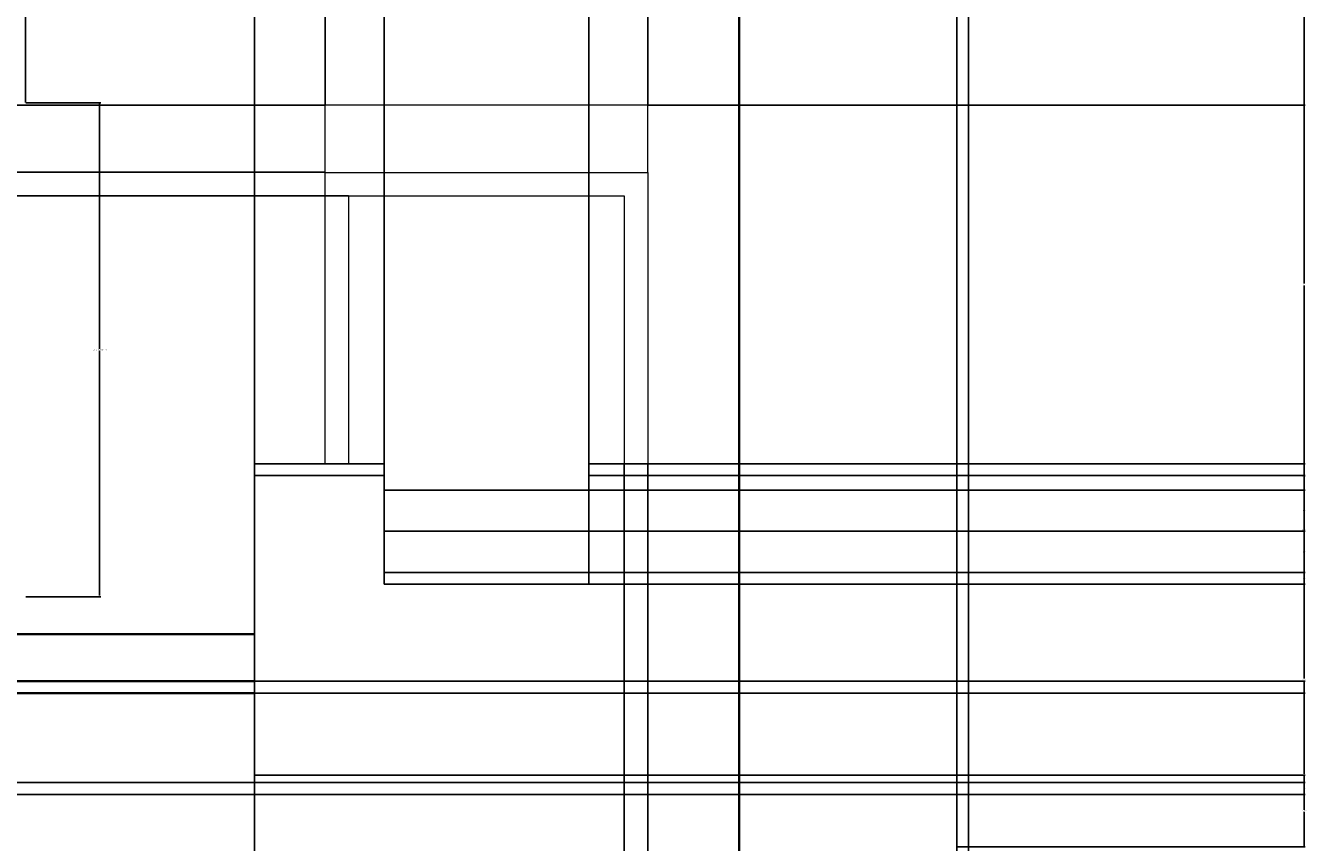
# Model space of a CAD drawing. Units: inches. Extents: x 1817 to 2378, y 1915 to 2370.
# Tile 7 of 8: x 2160 to 2378, y 2092 to 2231. Entities that reach past the tile are written whole.
import ezdxf

# ---------------------------------------------------------------- set-up
doc = ezdxf.new("R2010")
doc.units = ezdxf.units.IN
for name, color, linetype, lineweight in [('A-ANNO-DIMS', 2, 'Continuous', 18), ('A-ELEV', 7, 'Continuous', 35), ('A-ELEV-BALC', 3, 'Continuous', 25), ('A-GLAZ', 4, 'Continuous', 18)]:
    doc.layers.add(name, color=color, linetype=linetype, lineweight=lineweight)
doc.styles.get("Standard").update_dxf_attribs({"font": 'arial.ttf'})
doc.dimstyles.get("Standard").update_dxf_attribs({"dimtxt": 0.18, "dimasz": 0.18, "dimexe": 0.18, "dimexo": 0.0625, "dimgap": 0.09, "dimtad": 0, "dimtih": 1, "dimtoh": 1, "dimdec": 4, "dimzin": 0, "dimdsep": 46, "dimtxsty": 'Standard', "dimcen": 0.09, "dimadec": 0, "dimazin": 0, "dimtfac": 1, "dimtdec": 4, "dimtofl": 0, "dimtmove": 0, "dimatfit": 3, "dimfxl": 1, "dimtolj": 1, "dimtzin": 0, "dimarcsym": 0})

# ---------------------------------------------------------------- blocks, each defined once
blk = doc.blocks.new('*D8')
at = {"layer": 'A-ANNO-DIMS', "color": 0, "lineweight": -2, "transparency": 16777216}
for p, q in [((2159.68, 2217.9), (2172.4, 2217.9)), ((2172.22, 2217.72), (2172.22, 2176.08)), ((2172.22, 2134.08), (2172.22, 2175.71)), ((2159.68, 2133.9), (2172.4, 2133.9))]:
    blk.add_line(p, q, dxfattribs=at)
at = {"layer": 'A-ANNO-DIMS', "color": 0, "transparency": 16777216}
for points in [[(2172.19, 2217.72), (2172.25, 2217.72), (2172.22, 2217.9)], [(2172.19, 2134.08), (2172.25, 2134.08), (2172.22, 2133.9)]]:
    blk.add_solid(points, dxfattribs=at)
at = {"layer": 'Defpoints', "color": 0, "transparency": 16777216}
for p in [(2159.62, 2217.9), (2172.22, 2217.9), (2159.62, 2133.9)]:
    blk.add_point(p, dxfattribs=at)
at = {"layer": 'A-ANNO-DIMS', "color": 0, "transparency": 16777216, "insert": (2172.22, 2175.9), "char_height": 0.18, "attachment_point": 5}
blk.add_mtext('\\A1;TALL WINDOW 84 TYP.', dxfattribs=at)
blk = doc.blocks.new('*D23')
at = {"layer": 'A-ANNO-DIMS', "color": 0, "lineweight": -2, "transparency": 16777216}
for p, q in [((2320.11, 2156.45), (2320.11, 1915.08)), ((1867.08, 1965.45), (1867.08, 1915.08)), ((1867.26, 1915.26), (2093.3, 1915.26)), ((2319.93, 1915.26), (2093.89, 1915.26))]:
    blk.add_line(p, q, dxfattribs=at)
at = {"layer": 'A-ANNO-DIMS', "color": 0, "transparency": 16777216}
for points in [[(1867.26, 1915.29), (1867.26, 1915.23), (1867.08, 1915.26)], [(2319.93, 1915.29), (2319.93, 1915.23), (2320.11, 1915.26)]]:
    blk.add_solid(points, dxfattribs=at)
at = {"layer": 'Defpoints', "color": 0, "transparency": 16777216}
for p in [(2320.11, 2156.51), (1867.08, 1965.51), (2320.11, 1915.26)]:
    blk.add_point(p, dxfattribs=at)
at = {"layer": 'A-ANNO-DIMS', "color": 0, "transparency": 16777216, "insert": (2093.6, 1915.26), "char_height": 0.18, "attachment_point": 5}
blk.add_mtext('\\A1;453', dxfattribs=at)
blk = doc.blocks.new('*D24')
at = {"layer": 'A-ANNO-DIMS', "color": 0, "lineweight": -2, "transparency": 16777216}
for p, q in [((2198.59, 2103.51), (2198.59, 1915.08)), ((2318.11, 2103.51), (2318.11, 1915.08)), ((2198.77, 1915.26), (2257.89, 1915.26)), ((2317.93, 1915.26), (2258.8, 1915.26))]:
    blk.add_line(p, q, dxfattribs=at)
at = {"layer": 'A-ANNO-DIMS', "color": 0, "transparency": 16777216}
for points in [[(2198.77, 1915.29), (2198.77, 1915.23), (2198.59, 1915.26)], [(2317.93, 1915.29), (2317.93, 1915.23), (2318.11, 1915.26)]]:
    blk.add_solid(points, dxfattribs=at)
at = {"layer": 'Defpoints', "color": 0, "transparency": 16777216}
for p in [(2198.59, 2103.57), (2318.11, 2103.57), (2318.11, 1915.26)]:
    blk.add_point(p, dxfattribs=at)
at = {"layer": 'A-ANNO-DIMS', "color": 0, "transparency": 16777216, "insert": (2258.35, 1915.26), "char_height": 0.18, "attachment_point": 5}
blk.add_mtext('\\A1;119.52', dxfattribs=at)
blk = doc.blocks.new('*D36')
at = {"layer": 'A-ANNO-DIMS', "color": 0, "lineweight": -2, "transparency": 16777216}
for p, q in [((2159.62, 2217.96), (2159.62, 2369.94)), ((2159.8, 2369.76), (2178.71, 2369.76)), ((2198.41, 2369.76), (2179.5, 2369.76)), ((2198.59, 2156.58), (2198.59, 2369.94))]:
    blk.add_line(p, q, dxfattribs=at)
at = {"layer": 'A-ANNO-DIMS', "color": 0, "transparency": 16777216}
for points in [[(2159.8, 2369.79), (2159.8, 2369.73), (2159.62, 2369.76)], [(2198.41, 2369.79), (2198.41, 2369.73), (2198.59, 2369.76)]]:
    blk.add_solid(points, dxfattribs=at)
at = {"layer": 'Defpoints', "color": 0, "transparency": 16777216}
for p in [(2198.59, 2369.76), (2159.62, 2217.9), (2198.59, 2156.51)]:
    blk.add_point(p, dxfattribs=at)
at = {"layer": 'A-ANNO-DIMS', "color": 0, "transparency": 16777216, "insert": (2179.1, 2369.76), "char_height": 0.18, "attachment_point": 5}
blk.add_mtext('\\A1;38.97', dxfattribs=at)
blk = doc.blocks.new('*D37')
at = {"layer": 'A-ANNO-DIMS', "color": 0, "lineweight": -2, "transparency": 16777216}
for p, q in [((2198.59, 2156.58), (2198.59, 2369.94)), ((2198.77, 2369.76), (2204.15, 2369.76)), ((2210.44, 2369.76), (2205.06, 2369.76)), ((2210.62, 2217.57), (2210.62, 2369.94))]:
    blk.add_line(p, q, dxfattribs=at)
at = {"layer": 'A-ANNO-DIMS', "color": 0, "transparency": 16777216}
for points in [[(2198.77, 2369.79), (2198.77, 2369.73), (2198.59, 2369.76)], [(2210.44, 2369.79), (2210.44, 2369.73), (2210.62, 2369.76)]]:
    blk.add_solid(points, dxfattribs=at)
at = {"layer": 'Defpoints', "color": 0, "transparency": 16777216}
for p in [(2210.62, 2369.76), (2210.62, 2217.51), (2198.59, 2156.51)]:
    blk.add_point(p, dxfattribs=at)
at = {"layer": 'A-ANNO-DIMS', "color": 0, "transparency": 16777216, "insert": (2204.6, 2369.76), "char_height": 0.18, "attachment_point": 5}
blk.add_mtext('\\A1;12.027', dxfattribs=at)
blk = doc.blocks.new('*D38')
at = {"layer": 'A-ANNO-DIMS', "color": 0, "lineweight": -2, "transparency": 16777216}
for p, q in [((2210.62, 2217.57), (2210.62, 2369.94)), ((2210.8, 2369.76), (2215.41, 2369.76)), ((2220.44, 2369.76), (2215.83, 2369.76)), ((2220.62, 2136.11), (2220.62, 2369.94))]:
    blk.add_line(p, q, dxfattribs=at)
at = {"layer": 'A-ANNO-DIMS', "color": 0, "transparency": 16777216}
for points in [[(2210.8, 2369.79), (2210.8, 2369.73), (2210.62, 2369.76)], [(2220.44, 2369.79), (2220.44, 2369.73), (2220.62, 2369.76)]]:
    blk.add_solid(points, dxfattribs=at)
at = {"layer": 'Defpoints', "color": 0, "transparency": 16777216}
for p in [(2220.62, 2369.76), (2210.62, 2217.51), (2220.62, 2136.04)]:
    blk.add_point(p, dxfattribs=at)
at = {"layer": 'A-ANNO-DIMS', "color": 0, "transparency": 16777216, "insert": (2215.62, 2369.76), "char_height": 0.18, "attachment_point": 5}
blk.add_mtext('\\A1;10', dxfattribs=at)
blk = doc.blocks.new('*D39')
at = {"layer": 'A-ANNO-DIMS', "color": 0, "lineweight": -2, "transparency": 16777216}
for p, q in [((2220.62, 2136.11), (2220.62, 2369.94)), ((2220.8, 2369.76), (2237.66, 2369.76)), ((2255.31, 2369.76), (2238.45, 2369.76)), ((2255.49, 2136.11), (2255.49, 2369.94))]:
    blk.add_line(p, q, dxfattribs=at)
at = {"layer": 'A-ANNO-DIMS', "color": 0, "transparency": 16777216}
for points in [[(2220.8, 2369.79), (2220.8, 2369.73), (2220.62, 2369.76)], [(2255.31, 2369.79), (2255.31, 2369.73), (2255.49, 2369.76)]]:
    blk.add_solid(points, dxfattribs=at)
at = {"layer": 'Defpoints', "color": 0, "transparency": 16777216}
for p in [(2255.49, 2369.76), (2220.62, 2136.04), (2255.49, 2136.04)]:
    blk.add_point(p, dxfattribs=at)
at = {"layer": 'A-ANNO-DIMS', "color": 0, "transparency": 16777216, "insert": (2238.05, 2369.76), "char_height": 0.18, "attachment_point": 5}
blk.add_mtext('\\A1;34.87', dxfattribs=at)
blk = doc.blocks.new('*D40')
at = {"layer": 'A-ANNO-DIMS', "color": 0, "lineweight": -2, "transparency": 16777216}
for p, q in [((2255.49, 2136.11), (2255.49, 2369.94)), ((2255.67, 2369.76), (2260.28, 2369.76)), ((2265.31, 2369.76), (2260.7, 2369.76)), ((2265.49, 2217.57), (2265.49, 2369.94))]:
    blk.add_line(p, q, dxfattribs=at)
at = {"layer": 'A-ANNO-DIMS', "color": 0, "transparency": 16777216}
for points in [[(2255.67, 2369.79), (2255.67, 2369.73), (2255.49, 2369.76)], [(2265.31, 2369.79), (2265.31, 2369.73), (2265.49, 2369.76)]]:
    blk.add_solid(points, dxfattribs=at)
at = {"layer": 'Defpoints', "color": 0, "transparency": 16777216}
for p in [(2265.49, 2369.76), (2265.49, 2217.51), (2255.49, 2136.04)]:
    blk.add_point(p, dxfattribs=at)
at = {"layer": 'A-ANNO-DIMS', "color": 0, "transparency": 16777216, "insert": (2260.49, 2369.76), "char_height": 0.18, "attachment_point": 5}
blk.add_mtext('\\A1;10', dxfattribs=at)
blk = doc.blocks.new('*D41')
at = {"layer": 'A-ANNO-DIMS', "color": 0, "lineweight": -2, "transparency": 16777216}
for p, q in [((2318.11, 2103.63), (2318.11, 2369.94)), ((2318.29, 2369.76), (2318.96, 2369.76)), ((2319.93, 2369.76), (2319.26, 2369.76)), ((2320.11, 2156.58), (2320.11, 2369.94))]:
    blk.add_line(p, q, dxfattribs=at)
at = {"layer": 'A-ANNO-DIMS', "color": 0, "transparency": 16777216}
for points in [[(2318.29, 2369.79), (2318.29, 2369.73), (2318.11, 2369.76)], [(2319.93, 2369.79), (2319.93, 2369.73), (2320.11, 2369.76)]]:
    blk.add_solid(points, dxfattribs=at)
at = {"layer": 'Defpoints', "color": 0, "transparency": 16777216}
for p in [(2320.11, 2369.76), (2320.11, 2156.51), (2318.11, 2103.57)]:
    blk.add_point(p, dxfattribs=at)
at = {"layer": 'A-ANNO-DIMS', "color": 0, "transparency": 16777216, "insert": (2319.11, 2369.76), "char_height": 0.18, "attachment_point": 5}
blk.add_mtext('\\A1;2', dxfattribs=at)
blk = doc.blocks.new('*D52')
at = {"layer": 'A-ANNO-DIMS', "color": 0, "lineweight": -2, "transparency": 16777216}
for p, q in [((2198.65, 2119.51), (2377.4, 2119.51)), ((2377.22, 2119.33), (2377.22, 2118.69)), ((2198.65, 2117.51), (2377.4, 2117.51)), ((2377.22, 2117.69), (2377.22, 2118.33))]:
    blk.add_line(p, q, dxfattribs=at)
at = {"layer": 'A-ANNO-DIMS', "color": 0, "transparency": 16777216}
for points in [[(2377.19, 2119.33), (2377.25, 2119.33), (2377.22, 2119.51)], [(2377.19, 2117.69), (2377.25, 2117.69), (2377.22, 2117.51)]]:
    blk.add_solid(points, dxfattribs=at)
at = {"layer": 'Defpoints', "color": 0, "transparency": 16777216}
for p in [(2198.59, 2119.51), (2377.22, 2119.51), (2198.59, 2117.51)]:
    blk.add_point(p, dxfattribs=at)
at = {"layer": 'A-ANNO-DIMS', "color": 0, "transparency": 16777216, "insert": (2377.22, 2118.51), "char_height": 0.18, "attachment_point": 5}
blk.add_mtext('\\A1;2', dxfattribs=at)
blk = doc.blocks.new('*D71')
at = {"layer": 'A-ANNO-DIMS', "color": 0, "lineweight": -2, "transparency": 16777216}
for p, q in [((2318.17, 2103.57), (2377.4, 2103.57)), ((2377.22, 2103.39), (2377.22, 2097.65)), ((2377.22, 2091.54), (2377.22, 2097.29)), ((2318.17, 2091.36), (2377.4, 2091.36))]:
    blk.add_line(p, q, dxfattribs=at)
at = {"layer": 'A-ANNO-DIMS', "color": 0, "transparency": 16777216}
for points in [[(2377.19, 2103.39), (2377.25, 2103.39), (2377.22, 2103.57)], [(2377.19, 2091.54), (2377.25, 2091.54), (2377.22, 2091.36)]]:
    blk.add_solid(points, dxfattribs=at)
at = {"layer": 'Defpoints', "color": 0, "transparency": 16777216}
for p in [(2318.11, 2103.57), (2377.22, 2103.57), (2318.11, 2091.36)]:
    blk.add_point(p, dxfattribs=at)
at = {"layer": 'A-ANNO-DIMS', "color": 0, "transparency": 16777216, "insert": (2377.22, 2097.47), "char_height": 0.18, "attachment_point": 5}
blk.add_mtext('\\A1;12.207', dxfattribs=at)
blk = doc.blocks.new('*D72')
at = {"layer": 'A-ANNO-DIMS', "color": 0, "lineweight": -2, "transparency": 16777216}
for p, q in [((2220.68, 2136.04), (2377.4, 2136.04)), ((2377.22, 2135.86), (2377.22, 2119.99)), ((2377.22, 2103.75), (2377.22, 2119.63)), ((2318.17, 2103.57), (2377.4, 2103.57))]:
    blk.add_line(p, q, dxfattribs=at)
at = {"layer": 'A-ANNO-DIMS', "color": 0, "transparency": 16777216}
for points in [[(2377.19, 2135.86), (2377.25, 2135.86), (2377.22, 2136.04)], [(2377.19, 2103.75), (2377.25, 2103.75), (2377.22, 2103.57)]]:
    blk.add_solid(points, dxfattribs=at)
at = {"layer": 'Defpoints', "color": 0, "transparency": 16777216}
for p in [(2220.62, 2136.04), (2377.22, 2136.04), (2318.11, 2103.57)]:
    blk.add_point(p, dxfattribs=at)
at = {"layer": 'A-ANNO-DIMS', "color": 0, "transparency": 16777216, "insert": (2377.22, 2119.81), "char_height": 0.18, "attachment_point": 5}
blk.add_mtext('\\A1;32.47', dxfattribs=at)
blk = doc.blocks.new('*D73')
at = {"layer": 'A-ANNO-DIMS', "color": 0, "lineweight": -2, "transparency": 16777216}
for p, q in [((2320.17, 2154.51), (2377.4, 2154.51)), ((2377.22, 2154.33), (2377.22, 2145.46)), ((2377.22, 2136.22), (2377.22, 2145.1)), ((2220.68, 2136.04), (2377.4, 2136.04))]:
    blk.add_line(p, q, dxfattribs=at)
at = {"layer": 'A-ANNO-DIMS', "color": 0, "transparency": 16777216}
for points in [[(2377.19, 2154.33), (2377.25, 2154.33), (2377.22, 2154.51)], [(2377.19, 2136.22), (2377.25, 2136.22), (2377.22, 2136.04)]]:
    blk.add_solid(points, dxfattribs=at)
at = {"layer": 'Defpoints', "color": 0, "transparency": 16777216}
for p in [(2320.11, 2154.51), (2377.22, 2154.51), (2220.62, 2136.04)]:
    blk.add_point(p, dxfattribs=at)
at = {"layer": 'A-ANNO-DIMS', "color": 0, "transparency": 16777216, "insert": (2377.22, 2145.28), "char_height": 0.18, "attachment_point": 5}
blk.add_mtext('\\A1;18.47', dxfattribs=at)
blk = doc.blocks.new('*D74')
at = {"layer": 'A-ANNO-DIMS', "color": 0, "lineweight": -2, "transparency": 16777216}
for p, q in [((2320.17, 2156.51), (2377.4, 2156.51)), ((2377.22, 2156.33), (2377.22, 2155.69)), ((2320.17, 2154.51), (2377.4, 2154.51)), ((2377.22, 2154.69), (2377.22, 2155.33))]:
    blk.add_line(p, q, dxfattribs=at)
at = {"layer": 'A-ANNO-DIMS', "color": 0, "transparency": 16777216}
for points in [[(2377.19, 2156.33), (2377.25, 2156.33), (2377.22, 2156.51)], [(2377.19, 2154.69), (2377.25, 2154.69), (2377.22, 2154.51)]]:
    blk.add_solid(points, dxfattribs=at)
at = {"layer": 'Defpoints', "color": 0, "transparency": 16777216}
for p in [(2320.11, 2156.51), (2377.22, 2156.51), (2320.11, 2154.51)]:
    blk.add_point(p, dxfattribs=at)
at = {"layer": 'A-ANNO-DIMS', "color": 0, "transparency": 16777216, "insert": (2377.22, 2155.51), "char_height": 0.18, "attachment_point": 5}
blk.add_mtext('\\A1;2', dxfattribs=at)
blk = doc.blocks.new('*D75')
at = {"layer": 'A-ANNO-DIMS', "color": 0, "lineweight": -2, "transparency": 16777216}
for p, q in [((2265.55, 2217.51), (2377.4, 2217.51)), ((2377.22, 2217.33), (2377.22, 2187.19)), ((2377.22, 2156.69), (2377.22, 2186.83)), ((2320.17, 2156.51), (2377.4, 2156.51))]:
    blk.add_line(p, q, dxfattribs=at)
at = {"layer": 'A-ANNO-DIMS', "color": 0, "transparency": 16777216}
for points in [[(2377.19, 2217.33), (2377.25, 2217.33), (2377.22, 2217.51)], [(2377.19, 2156.69), (2377.25, 2156.69), (2377.22, 2156.51)]]:
    blk.add_solid(points, dxfattribs=at)
at = {"layer": 'Defpoints', "color": 0, "transparency": 16777216}
for p in [(2265.49, 2217.51), (2377.22, 2217.51), (2320.11, 2156.51)]:
    blk.add_point(p, dxfattribs=at)
at = {"layer": 'A-ANNO-DIMS', "color": 0, "transparency": 16777216, "insert": (2377.22, 2187.01), "char_height": 0.18, "attachment_point": 5}
blk.add_mtext('\\A1;61', dxfattribs=at)
blk = doc.blocks.new('*D76')
at = {"layer": 'A-ANNO-DIMS', "color": 0, "lineweight": -2, "transparency": 16777216}
for p, q in [((2281.147352, 2261.508728), (2377.398057, 2261.508728)), ((2377.218057, 2261.328728), (2377.218057, 2239.688728)), ((2377.218057, 2217.688728), (2377.218057, 2239.328728)), ((2265.550872, 2217.508728), (2377.398057, 2217.508728))]:
    blk.add_line(p, q, dxfattribs=at)
at = {"layer": 'A-ANNO-DIMS', "color": 0, "transparency": 16777216}
for points in [[(2377.188057, 2261.328728), (2377.248057, 2261.328728), (2377.218057, 2261.508728)], [(2377.188057, 2217.688728), (2377.248057, 2217.688728), (2377.218057, 2217.508728)]]:
    blk.add_solid(points, dxfattribs=at)
at = {"layer": 'Defpoints', "color": 0, "transparency": 16777216}
for p in [(2281.084852, 2261.508728), (2377.218057, 2261.508728), (2265.488372, 2217.508728)]:
    blk.add_point(p, dxfattribs=at)
at = {"layer": 'A-ANNO-DIMS', "color": 0, "transparency": 16777216, "insert": (2377.218057, 2239.508728), "char_height": 0.18, "attachment_point": 5}
blk.add_mtext('\\A1;44', dxfattribs=at)
blk = doc.blocks.new('*D81')
at = {"layer": 'A-ANNO-DIMS', "color": 0, "lineweight": -2, "transparency": 16777216}
for p, q in [((2198.53, 2117.51), (1817.4, 2117.51)), ((1817.58, 2117.33), (1817.58, 2105.16)), ((1817.58, 2092.63), (1817.58, 2104.8)), ((2123.56, 2092.45), (1817.4, 2092.45))]:
    blk.add_line(p, q, dxfattribs=at)
at = {"layer": 'A-ANNO-DIMS', "color": 0, "transparency": 16777216}
for points in [[(1817.55, 2117.33), (1817.61, 2117.33), (1817.58, 2117.51)], [(1817.55, 2092.63), (1817.61, 2092.63), (1817.58, 2092.45)]]:
    blk.add_solid(points, dxfattribs=at)
at = {"layer": 'Defpoints', "color": 0, "transparency": 16777216}
for p in [(1817.58, 2117.51), (2198.59, 2117.51), (2123.62, 2092.45)]:
    blk.add_point(p, dxfattribs=at)
at = {"layer": 'A-ANNO-DIMS', "color": 0, "transparency": 16777216, "insert": (1817.58, 2104.98), "char_height": 0.18, "attachment_point": 5}
blk.add_mtext('\\A1;25.06', dxfattribs=at)
blk = doc.blocks.new('*D82')
at = {"layer": 'A-ANNO-DIMS', "color": 0, "lineweight": -2, "transparency": 16777216}
for p, q in [((2123.56, 2133.9), (1817.4, 2133.9)), ((1817.58, 2133.72), (1817.58, 2130.88)), ((1817.58, 2127.69), (1817.58, 2130.52)), ((2198.53, 2127.51), (1817.4, 2127.51))]:
    blk.add_line(p, q, dxfattribs=at)
at = {"layer": 'A-ANNO-DIMS', "color": 0, "transparency": 16777216}
for points in [[(1817.55, 2133.72), (1817.61, 2133.72), (1817.58, 2133.9)], [(1817.55, 2127.69), (1817.61, 2127.69), (1817.58, 2127.51)]]:
    blk.add_solid(points, dxfattribs=at)
at = {"layer": 'Defpoints', "color": 0, "transparency": 16777216}
for p in [(1817.58, 2133.9), (2123.62, 2133.9), (2198.59, 2127.51)]:
    blk.add_point(p, dxfattribs=at)
at = {"layer": 'A-ANNO-DIMS', "color": 0, "transparency": 16777216, "insert": (1817.58, 2130.7), "char_height": 0.18, "attachment_point": 5}
blk.add_mtext('\\A1;6.387', dxfattribs=at)
blk = doc.blocks.new('*D89')
at = {"layer": 'A-ANNO-DIMS', "color": 0, "lineweight": -2, "transparency": 16777216}
for p, q in [((1944.89, 2102.28), (2377.4, 2102.28)), ((2377.22, 2102.1), (2377.22, 2101.46)), ((1946.89, 2100.28), (2377.4, 2100.28)), ((2377.22, 2100.46), (2377.22, 2101.09))]:
    blk.add_line(p, q, dxfattribs=at)
at = {"layer": 'A-ANNO-DIMS', "color": 0, "transparency": 16777216}
for points in [[(2377.19, 2102.1), (2377.25, 2102.1), (2377.22, 2102.28)], [(2377.19, 2100.46), (2377.25, 2100.46), (2377.22, 2100.28)]]:
    blk.add_solid(points, dxfattribs=at)
at = {"layer": 'Defpoints', "color": 0, "transparency": 16777216}
for p in [(1944.83, 2102.28), (2377.22, 2102.28), (1946.83, 2100.28)]:
    blk.add_point(p, dxfattribs=at)
at = {"layer": 'A-ANNO-DIMS', "color": 0, "transparency": 16777216, "insert": (2377.22, 2101.28), "char_height": 0.18, "attachment_point": 5}
blk.add_mtext('\\A1;2.00', dxfattribs=at)
blk = doc.blocks.new('*D100')
at = {"layer": 'A-ANNO-DIMS', "color": 0, "lineweight": -2, "transparency": 16777216}
for p, q in [((2255.55, 2156.51), (2377.4, 2156.51)), ((2377.22, 2156.33), (2377.22, 2154.46)), ((2377.22, 2152.22), (2377.22, 2154.1)), ((2255.55, 2152.04), (2377.4, 2152.04))]:
    blk.add_line(p, q, dxfattribs=at)
at = {"layer": 'A-ANNO-DIMS', "color": 0, "transparency": 16777216}
for points in [[(2377.19, 2156.33), (2377.25, 2156.33), (2377.22, 2156.51)], [(2377.19, 2152.22), (2377.25, 2152.22), (2377.22, 2152.04)]]:
    blk.add_solid(points, dxfattribs=at)
at = {"layer": 'Defpoints', "color": 0, "transparency": 16777216}
for p in [(2255.49, 2156.51), (2255.49, 2152.04), (2377.22, 2152.04)]:
    blk.add_point(p, dxfattribs=at)
at = {"layer": 'A-ANNO-DIMS', "color": 0, "transparency": 16777216, "insert": (2377.22, 2154.28), "char_height": 0.18, "attachment_point": 5}
blk.add_mtext('\\A1;4.471', dxfattribs=at)
blk = doc.blocks.new('*D101')
at = {"layer": 'A-ANNO-DIMS', "color": 0, "lineweight": -2, "transparency": 16777216}
for p, q in [((2255.55, 2152.04), (2377.4, 2152.04)), ((2377.22, 2151.86), (2377.22, 2148.72)), ((2377.22, 2145.22), (2377.22, 2148.36)), ((2255.55, 2145.04), (2377.4, 2145.04))]:
    blk.add_line(p, q, dxfattribs=at)
at = {"layer": 'A-ANNO-DIMS', "color": 0, "transparency": 16777216}
for points in [[(2377.19, 2151.86), (2377.25, 2151.86), (2377.22, 2152.04)], [(2377.19, 2145.22), (2377.25, 2145.22), (2377.22, 2145.04)]]:
    blk.add_solid(points, dxfattribs=at)
at = {"layer": 'Defpoints', "color": 0, "transparency": 16777216}
for p in [(2255.49, 2152.04), (2255.49, 2145.04), (2377.22, 2145.04)]:
    blk.add_point(p, dxfattribs=at)
at = {"layer": 'A-ANNO-DIMS', "color": 0, "transparency": 16777216, "insert": (2377.22, 2148.54), "char_height": 0.18, "attachment_point": 5}
blk.add_mtext('\\A1;7.00', dxfattribs=at)
blk = doc.blocks.new('*D102')
at = {"layer": 'A-ANNO-DIMS', "color": 0, "lineweight": -2, "transparency": 16777216}
for p, q in [((2255.55, 2145.04), (2377.4, 2145.04)), ((2377.22, 2144.86), (2377.22, 2141.72)), ((2377.22, 2138.22), (2377.22, 2141.36)), ((2255.55, 2138.04), (2377.4, 2138.04))]:
    blk.add_line(p, q, dxfattribs=at)
at = {"layer": 'A-ANNO-DIMS', "color": 0, "transparency": 16777216}
for points in [[(2377.19, 2144.86), (2377.25, 2144.86), (2377.22, 2145.04)], [(2377.19, 2138.22), (2377.25, 2138.22), (2377.22, 2138.04)]]:
    blk.add_solid(points, dxfattribs=at)
at = {"layer": 'Defpoints', "color": 0, "transparency": 16777216}
for p in [(2255.49, 2145.04), (2255.49, 2138.04), (2377.22, 2138.04)]:
    blk.add_point(p, dxfattribs=at)
at = {"layer": 'A-ANNO-DIMS', "color": 0, "transparency": 16777216, "insert": (2377.22, 2141.54), "char_height": 0.18, "attachment_point": 5}
blk.add_mtext('\\A1;7.00', dxfattribs=at)
blk = doc.blocks.new('*D103')
at = {"layer": 'A-ANNO-DIMS', "color": 0, "lineweight": -2, "transparency": 16777216}
for p, q in [((2255.55, 2138.04), (2377.4, 2138.04)), ((2377.22, 2137.86), (2377.22, 2137.22)), ((2377.22, 2136.22), (2377.22, 2136.86)), ((2255.55, 2136.04), (2377.4, 2136.04))]:
    blk.add_line(p, q, dxfattribs=at)
at = {"layer": 'A-ANNO-DIMS', "color": 0, "transparency": 16777216}
for points in [[(2377.19, 2137.86), (2377.25, 2137.86), (2377.22, 2138.04)], [(2377.19, 2136.22), (2377.25, 2136.22), (2377.22, 2136.04)]]:
    blk.add_solid(points, dxfattribs=at)
at = {"layer": 'Defpoints', "color": 0, "transparency": 16777216}
for p in [(2255.49, 2138.04), (2255.49, 2136.04), (2377.22, 2136.04)]:
    blk.add_point(p, dxfattribs=at)
at = {"layer": 'A-ANNO-DIMS', "color": 0, "transparency": 16777216, "insert": (2377.22, 2137.04), "char_height": 0.18, "attachment_point": 5}
blk.add_mtext('\\A1;2.00', dxfattribs=at)
blk = doc.blocks.new('*D104')
at = {"layer": 'A-ANNO-DIMS', "color": 0, "lineweight": -2, "transparency": 16777216}
for p, q in [((2210.55, 2217.51), (1817.4, 2217.51)), ((1817.58, 2217.33), (1817.58, 2211.97)), ((1817.58, 2206.26), (1817.58, 2211.61)), ((2210.55, 2206.08), (1817.4, 2206.08))]:
    blk.add_line(p, q, dxfattribs=at)
at = {"layer": 'A-ANNO-DIMS', "color": 0, "transparency": 16777216}
for points in [[(1817.55, 2217.33), (1817.61, 2217.33), (1817.58, 2217.51)], [(1817.55, 2206.26), (1817.61, 2206.26), (1817.58, 2206.08)]]:
    blk.add_solid(points, dxfattribs=at)
at = {"layer": 'Defpoints', "color": 0, "transparency": 16777216}
for p in [(2210.62, 2217.51), (1817.58, 2206.08), (2210.62, 2206.08)]:
    blk.add_point(p, dxfattribs=at)
at = {"layer": 'A-ANNO-DIMS', "color": 0, "transparency": 16777216, "insert": (1817.58, 2211.79), "char_height": 0.18, "attachment_point": 5}
blk.add_mtext('\\A1;11.433', dxfattribs=at)
blk = doc.blocks.new('*D105')
at = {"layer": 'A-ANNO-DIMS', "color": 0, "lineweight": -2, "transparency": 16777216}
for p, q in [((2210.55, 2206.08), (1817.4, 2206.08)), ((1817.58, 2205.9), (1817.58, 2204.26)), ((1817.58, 2202.26), (1817.58, 2203.89)), ((2214.55, 2202.08), (1817.4, 2202.08))]:
    blk.add_line(p, q, dxfattribs=at)
at = {"layer": 'A-ANNO-DIMS', "color": 0, "transparency": 16777216}
for points in [[(1817.55, 2205.9), (1817.61, 2205.9), (1817.58, 2206.08)], [(1817.55, 2202.26), (1817.61, 2202.26), (1817.58, 2202.08)]]:
    blk.add_solid(points, dxfattribs=at)
at = {"layer": 'Defpoints', "color": 0, "transparency": 16777216}
for p in [(2210.62, 2206.08), (1817.58, 2202.08), (2214.62, 2202.08)]:
    blk.add_point(p, dxfattribs=at)
at = {"layer": 'A-ANNO-DIMS', "color": 0, "transparency": 16777216, "insert": (1817.58, 2204.08), "char_height": 0.18, "attachment_point": 5}
blk.add_mtext('\\A1;4.00', dxfattribs=at)
blk = doc.blocks.new('*D106')
at = {"layer": 'A-ANNO-DIMS', "color": 0, "lineweight": -2, "transparency": 16777216}
for p, q in [((2261.49, 2156.45), (2261.49, 1915.08)), ((2265.49, 2156.45), (2265.49, 1915.08)), ((2261.67, 1915.26), (2263.16, 1915.26)), ((2265.31, 1915.26), (2263.82, 1915.26))]:
    blk.add_line(p, q, dxfattribs=at)
at = {"layer": 'A-ANNO-DIMS', "color": 0, "transparency": 16777216}
for points in [[(2261.67, 1915.29), (2261.67, 1915.23), (2261.49, 1915.26)], [(2265.31, 1915.29), (2265.31, 1915.23), (2265.49, 1915.26)]]:
    blk.add_solid(points, dxfattribs=at)
at = {"layer": 'Defpoints', "color": 0, "transparency": 16777216}
for p in [(2261.49, 2156.51), (2265.49, 2156.51), (2261.49, 1915.26)]:
    blk.add_point(p, dxfattribs=at)
at = {"layer": 'A-ANNO-DIMS', "color": 0, "transparency": 16777216, "insert": (2263.49, 1915.26), "char_height": 0.18, "attachment_point": 5}
blk.add_mtext('\\A1;4.00', dxfattribs=at)
blk = doc.blocks.new('*D119')
at = {"layer": 'A-ANNO-DIMS', "color": 0, "lineweight": -2, "transparency": 16777216}
for p, q in [((1903.08, 1989.57), (1903.08, 2369.94)), ((1903.26, 2369.76), (2091.62, 2369.76)), ((2280.9, 2369.76), (2092.55, 2369.76)), ((2281.08, 1989.57), (2281.08, 2369.94))]:
    blk.add_line(p, q, dxfattribs=at)
at = {"layer": 'A-ANNO-DIMS', "color": 0, "transparency": 16777216}
for points in [[(1903.26, 2369.79), (1903.26, 2369.73), (1903.08, 2369.76)], [(2280.9, 2369.79), (2280.9, 2369.73), (2281.08, 2369.76)]]:
    blk.add_solid(points, dxfattribs=at)
at = {"layer": 'Defpoints', "color": 0, "transparency": 16777216}
for p in [(2281.08, 2369.76), (1903.08, 1989.51), (2281.08, 1989.51)]:
    blk.add_point(p, dxfattribs=at)
at = {"layer": 'A-ANNO-DIMS', "color": 0, "transparency": 16777216, "insert": (2092.08, 2369.76), "char_height": 0.18, "attachment_point": 5}
blk.add_mtext('\\A1;378.00', dxfattribs=at)

msp = doc.modelspace()

# ---------------------------------------------------------------- linework, layer by layer
at = {"layer": 'A-ELEV'}
for p, q in [((2281.0849, 2251.5087), (2281.0849, 1965.5087)), ((2198.5896, 2127.5087), (1903.0849, 2127.5087)), ((2198.5896, 2119.5087), (1895.6961, 2119.5087)), ((2198.5896, 2117.5087), (1895.6961, 2117.5087))]:
    msp.add_line(p, q, dxfattribs=at)
at = {"layer": 'A-ELEV-BALC'}
for p, q in [((2198.5896, 2103.5721), (2198.5896, 2156.5133)), ((2198.5896, 2156.5133), (2220.6163, 2156.5133)), ((2220.6163, 2136.0427), (2220.6163, 2156.5133)), ((2255.4884, 2156.5133), (2255.4884, 2136.0427)), ((2255.4884, 2156.5133), (2320.1054, 2156.5133)), ((2320.1054, 2156.5133), (2320.1054, 2154.5133)), ((2198.5896, 2154.5133), (2220.6163, 2154.5133)), ((2255.4884, 2154.5133), (2320.1054, 2154.5133)), ((2318.1054, 2154.5133), (2318.1054, 2103.5721)), ((2255.4884, 2152.0427), (2220.6163, 2152.0427)), ((2255.4884, 2145.0427), (2220.6163, 2145.0427)), ((2255.4884, 2138.0427), (2220.6163, 2138.0427)), ((2255.4884, 2136.0427), (2220.6163, 2136.0427)), ((2318.1054, 2103.5721), (2198.5896, 2103.5721))]:
    msp.add_line(p, q, dxfattribs=at)
at = {"layer": 'A-GLAZ'}
for p, q in [((2210.6163, 2206.0753), (2210.6163, 2217.5087)), ((2265.4884, 2217.5087), (2210.6163, 2217.5087)), ((2265.4884, 2206.0753), (2265.4884, 2217.5087)), ((2210.6163, 2206.0753), (2265.4884, 2206.0753)), ((2210.6163, 2156.5133), (2210.6163, 2206.0753)), ((2210.6163, 2206.0753), (2265.4884, 2206.0753)), ((2265.4884, 2206.0753), (2265.4884, 2156.5133)), ((2214.6163, 2202.0753), (2261.4884, 2202.0753)), ((2214.6163, 2156.5133), (2214.6163, 2202.0753)), ((2261.4884, 2202.0753), (2261.4884, 2156.5133))]:
    msp.add_line(p, q, dxfattribs=at)

# ---------------------------------------------------------------- dimensions: what is measured, and where the dimension line sits
at = {"layer": 'A-ANNO-DIMS'}
for base, p1, p2, override, picture, middle in [((2281.0849, 2369.7587), (1903.0849, 1989.5087), (2281.0849, 1989.5087), {"dimdec": 2, "dimlfac": 1, "dimrnd": 0, "dimzin": 0, "dimdsep": 46, "dimlunit": 2}, '*D119', (2092.0849, 2369.7587)), ((2198.5896, 2369.7587), (2159.6179, 2217.8955), (2198.5896, 2156.5133), {"dimdec": 2, "dimlfac": 1, "dimrnd": 0, "dimzin": 0, "dimdsep": 46, "dimlunit": 2}, '*D36', (2179.1037, 2369.7587)), ((2210.6163, 2369.7587), (2198.5896, 2156.5133), (2210.6163, 2217.5087), {"dimdec": 3, "dimlfac": 1, "dimrnd": 0, "dimzin": 0, "dimdsep": 46, "dimlunit": 2}, '*D37', (2204.6029, 2369.7587)), ((2220.6163, 2369.7587), (2210.6163, 2217.5087), (2220.6163, 2136.0427), {"dimdec": 0, "dimlfac": 1, "dimrnd": 0, "dimzin": 0, "dimdsep": 46, "dimlunit": 2}, '*D38', (2215.6163, 2369.7587)), ((2255.4884, 2369.7587), (2220.6163, 2136.0427), (2255.4884, 2136.0427), {"dimdec": 2, "dimlfac": 1, "dimrnd": 0, "dimzin": 0, "dimdsep": 46, "dimlunit": 2}, '*D39', (2238.0523, 2369.7587)), ((2265.4884, 2369.7587), (2255.4884, 2136.0427), (2265.4884, 2217.5087), {"dimdec": 0, "dimlfac": 1, "dimrnd": 0, "dimzin": 0, "dimdsep": 46, "dimlunit": 2}, '*D40', (2260.4884, 2369.7587)), ((2320.1054, 2369.7587), (2318.1054, 2103.5721), (2320.1054, 2156.5133), {"dimdec": 0, "dimlfac": 1, "dimrnd": 0, "dimzin": 0, "dimdsep": 46, "dimlunit": 2}, '*D41', (2319.1054, 2369.7587)), ((2320.1054, 1915.2587), (1867.0849, 1965.5087), (2320.1054, 2156.5133), {"dimdec": 0, "dimlfac": 1, "dimrnd": 0, "dimzin": 0, "dimdsep": 46, "dimlunit": 2}, '*D23', (2093.5951, 1915.2587)), ((2261.4884, 1915.2587), (2265.4884, 2156.5133), (2261.4884, 2156.5133), {"dimdec": 2, "dimlfac": 1, "dimrnd": 0, "dimzin": 0, "dimdsep": 46, "dimlunit": 2}, '*D106', (2263.4884, 1915.2587)), ((2318.1054, 1915.2587), (2198.5896, 2103.5721), (2318.1054, 2103.5721), {"dimdec": 2, "dimlfac": 1, "dimrnd": 0, "dimzin": 0, "dimdsep": 46, "dimlunit": 2}, '*D24', (2258.3475, 1915.2587))]:
    dim = msp.add_linear_dim(base=base, p1=p1, p2=p2, dimstyle='Standard', override=override, dxfattribs=at)
    dim.commit()
    dim.dimension.update_dxf_attribs({"geometry": picture, "text_midpoint": middle})
for base, p1, p2, override, picture, middle in [((2377.2181, 2261.5087), (2265.4884, 2217.5087), (2281.0849, 2261.5087), {"dimdec": 0, "dimlfac": 1, "dimrnd": 0, "dimzin": 0, "dimdsep": 46, "dimlunit": 2}, '*D76', (2377.2181, 2239.5087)), ((1817.584, 2206.0753), (2210.6163, 2217.5087), (2210.6163, 2206.0753), {"dimdec": 3, "dimlfac": 1, "dimrnd": 0, "dimzin": 0, "dimdsep": 46, "dimlunit": 2}, '*D104', (1817.584, 2211.792)), ((2377.2181, 2217.5087), (2320.1054, 2156.5133), (2265.4884, 2217.5087), {"dimdec": 0, "dimlfac": 1, "dimrnd": 0, "dimzin": 0, "dimdsep": 46, "dimlunit": 2}, '*D75', (2377.2181, 2187.011)), ((1817.584, 2202.0753), (2210.6163, 2206.0753), (2214.6163, 2202.0753), {"dimdec": 2, "dimlfac": 1, "dimrnd": 0, "dimzin": 0, "dimdsep": 46, "dimlunit": 2}, '*D105', (1817.584, 2204.0753)), ((2377.2181, 2152.0427), (2255.4884, 2156.5133), (2255.4884, 2152.0427), {"dimdec": 3, "dimlfac": 1, "dimrnd": 0, "dimzin": 0, "dimdsep": 46, "dimlunit": 2}, '*D100', (2377.2181, 2154.278)), ((2377.2181, 2156.5133), (2320.1054, 2154.5133), (2320.1054, 2156.5133), {"dimdec": 0, "dimlfac": 1, "dimrnd": 0, "dimzin": 0, "dimdsep": 46, "dimlunit": 2}, '*D74', (2377.2181, 2155.5133)), ((2377.2181, 2154.5133), (2220.6163, 2136.0427), (2320.1054, 2154.5133), {"dimdec": 2, "dimlfac": 1, "dimrnd": 0, "dimzin": 0, "dimdsep": 46, "dimlunit": 2}, '*D73', (2377.2181, 2145.278)), ((2377.2181, 2145.0427), (2255.4884, 2152.0427), (2255.4884, 2145.0427), {"dimdec": 2, "dimlfac": 1, "dimrnd": 0, "dimzin": 0, "dimdsep": 46, "dimlunit": 2}, '*D101', (2377.2181, 2148.5427)), ((2377.2181, 2138.0427), (2255.4884, 2145.0427), (2255.4884, 2138.0427), {"dimdec": 2, "dimlfac": 1, "dimrnd": 0, "dimzin": 0, "dimdsep": 46, "dimlunit": 2}, '*D102', (2377.2181, 2141.5427)), ((2377.2181, 2136.0427), (2255.4884, 2138.0427), (2255.4884, 2136.0427), {"dimdec": 2, "dimlfac": 1, "dimrnd": 0, "dimzin": 0, "dimdsep": 46, "dimlunit": 2}, '*D103', (2377.2181, 2137.0427)), ((2377.2181, 2136.0427), (2318.1054, 2103.5721), (2220.6163, 2136.0427), {"dimdec": 2, "dimlfac": 1, "dimrnd": 0, "dimzin": 0, "dimdsep": 46, "dimlunit": 2}, '*D72', (2377.2181, 2119.8074)), ((1817.584, 2133.8955), (2198.5896, 2127.5087), (2123.6179, 2133.8955), {"dimdec": 3, "dimlfac": 1, "dimrnd": 0, "dimzin": 0, "dimdsep": 46, "dimlunit": 2}, '*D82', (1817.584, 2130.7021)), ((2377.2181, 2119.5087), (2198.5896, 2117.5087), (2198.5896, 2119.5087), {"dimdec": 0, "dimlfac": 1, "dimrnd": 0, "dimzin": 0, "dimdsep": 46, "dimlunit": 2}, '*D52', (2377.2181, 2118.5087)), ((1817.584, 2117.5087), (2123.6179, 2092.4468), (2198.5896, 2117.5087), {"dimdec": 2, "dimlfac": 1, "dimrnd": 0, "dimzin": 0, "dimdsep": 46, "dimlunit": 2}, '*D81', (1817.584, 2104.9777)), ((2377.2181, 2103.5721), (2318.1054, 2091.3647), (2318.1054, 2103.5721), {"dimdec": 3, "dimlfac": 1, "dimrnd": 0, "dimzin": 0, "dimdsep": 46, "dimlunit": 2}, '*D71', (2377.2181, 2097.4684)), ((2377.2181, 2102.2756), (1946.8265, 2100.2756), (1944.8265, 2102.2756), {"dimdec": 2, "dimlfac": 1, "dimrnd": 0, "dimzin": 0, "dimdsep": 46, "dimlunit": 2}, '*D89', (2377.2181, 2101.2756))]:
    dim = msp.add_linear_dim(base=base, p1=p1, p2=p2, angle=90, dimstyle='Standard', override=override, dxfattribs=at)
    dim.commit()
    dim.dimension.update_dxf_attribs({"geometry": picture, "text_midpoint": middle})
dim = msp.add_linear_dim(base=(2172.2179, 2217.8955), p1=(2159.6179, 2133.8955), p2=(2159.6179, 2217.8955), angle=90, text='TALL WINDOW <> TYP.', dimstyle='Standard', override={"dimdec": 0, "dimlfac": 1, "dimrnd": 0, "dimzin": 0, "dimdsep": 46, "dimlunit": 2}, dxfattribs=at)
dim.commit()
dim.dimension.update_dxf_attribs({"geometry": '*D8', "text_midpoint": (2172.2179, 2175.8955)})

doc.saveas('drawing.dxf')
